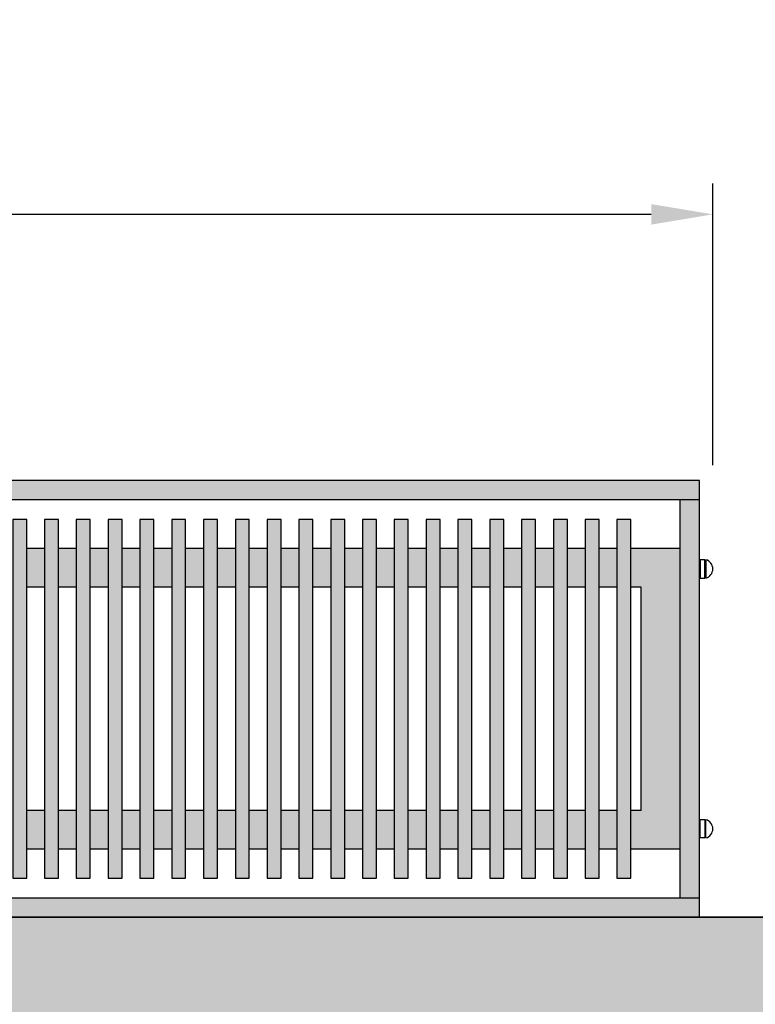
# Model space of a CAD drawing. Units: inches. Extents: x 3592 to 4861, y 1650 to 2243.
# Tile 14 of 30: x 4335 to 4365, y 1772 to 1812. Entities that reach past the tile are written whole.
import ezdxf

# ---------------------------------------------------------------- set-up
doc = ezdxf.new("R2010")
doc.units = ezdxf.units.IN
for name, color, linetype, lineweight in [('A-ANNO-DIMS', 2, 'Continuous', 13), ('A-FURN', 9, 'Continuous', 13), ('A-WALL', 7, 'Continuous', 35), ('estofado', 7, 'Continuous', 25)]:
    doc.layers.add(name, color=color, linetype=linetype, lineweight=lineweight)
doc.layers.add('A-WALL-PATT', color=252, linetype='Continuous', lineweight=13, true_color=0x939598)
doc.layers.add('MOBIL', color=7, linetype='Continuous')
doc.styles.get("Standard").update_dxf_attribs({"font": 'arial.ttf'})
doc.dimstyles.new('ISO-25', dxfattribs={"dimtxt": 9, "dimasz": 2.5, "dimexe": 1.25, "dimexo": 0.625, "dimtad": 1, "dimlunit": 3, "dimtxsty": 'Standard', "dimcen": 2.5, "dimadec": 0, "dimazin": 0, "dimtfac": 1, "dimtmove": 0, "dimatfit": 3, "dimfxl": 1, "dimarcsym": 0})

# ---------------------------------------------------------------- blocks, each defined once
blk = doc.blocks.new('Aparador Aido WV')
at = {"layer": 'MOBIL'}
h = blk.add_hatch(color=256, dxfattribs=at)
h.set_gradient(color1=(226, 228, 228), one_color=1, tint=1, name='CYLINDER')
h.paths.add_polyline_path([(0.9, -0.02), (0.9, 0), (-0.9, 0), (-0.9, -0.02)])
h = blk.add_hatch(color=256, dxfattribs=at)
h.set_gradient(color1=(226, 228, 228), one_color=1, tint=1)
h.paths.add_polyline_path([(-0.88, -0.02), (-0.9, -0.02), (-0.9, -0.43), (-0.88, -0.43)])
h = blk.add_hatch(color=256, dxfattribs=at)
h.set_gradient(color1=(106, 79, 62), color2=(55, 41, 32), one_color=1, tint=0.17)
h.paths.add_polyline_path([(-0.8151, -0.0402), (-0.8295, -0.0402), (-0.8295, -0.4098), (-0.8151, -0.4098)])
h = blk.add_hatch(color=256, dxfattribs=at)
h.set_gradient(color1=(106, 79, 62), color2=(55, 41, 32), one_color=1, tint=0.17)
h.paths.add_polyline_path([(-0.7967, -0.0402), (-0.7967, -0.4098), (-0.7823, -0.4098), (-0.7823, -0.0402)])
h = blk.add_hatch(color=256, dxfattribs=at)
h.set_gradient(color1=(106, 79, 62), color2=(55, 41, 32), one_color=1, tint=0.17)
h.paths.add_polyline_path([(-0.764, -0.0402), (-0.764, -0.4098), (-0.7496, -0.4098), (-0.7496, -0.0402)])
h = blk.add_hatch(color=256, dxfattribs=at)
h.set_gradient(color1=(106, 79, 62), color2=(55, 41, 32), one_color=1, tint=0.17)
h.paths.add_polyline_path([(-0.7312, -0.0402), (-0.7312, -0.4098), (-0.7168, -0.4098), (-0.7168, -0.0402)])
h = blk.add_hatch(color=256, dxfattribs=at)
h.set_gradient(color1=(106, 79, 62), color2=(55, 41, 32), one_color=1, tint=0.17)
h.paths.add_polyline_path([(-0.6985, -0.0402), (-0.6985, -0.4098), (-0.6841, -0.4098), (-0.6841, -0.0402)])
h = blk.add_hatch(color=256, dxfattribs=at)
h.set_gradient(color1=(106, 79, 62), color2=(55, 41, 32), one_color=1, tint=0.17)
h.paths.add_polyline_path([(-0.6657, -0.0402), (-0.6657, -0.4098), (-0.6513, -0.4098), (-0.6513, -0.0402)])
h = blk.add_hatch(color=256, dxfattribs=at)
h.set_gradient(color1=(106, 79, 62), color2=(55, 41, 32), one_color=1, tint=0.17)
h.paths.add_polyline_path([(-0.633, -0.0402), (-0.633, -0.4098), (-0.6186, -0.4098), (-0.6186, -0.0402)])
h = blk.add_hatch(color=256, dxfattribs=at)
h.set_gradient(color1=(106, 79, 62), color2=(55, 41, 32), one_color=1, tint=0.17)
h.paths.add_polyline_path([(-0.6002, -0.0402), (-0.6002, -0.4098), (-0.5858, -0.4098), (-0.5858, -0.0402)])
h = blk.add_hatch(color=256, dxfattribs=at)
h.set_gradient(color1=(106, 79, 62), color2=(55, 41, 32), one_color=1, tint=0.17)
h.paths.add_polyline_path([(-0.5675, -0.4098), (-0.5531, -0.4098), (-0.5531, -0.0402), (-0.5675, -0.0402)])
h = blk.add_hatch(color=256, dxfattribs=at)
h.set_gradient(color1=(106, 79, 62), color2=(55, 41, 32), one_color=1, tint=0.17)
h.paths.add_polyline_path([(-0.5347, -0.0402), (-0.5347, -0.4098), (-0.5203, -0.4098), (-0.5203, -0.0402)])
h = blk.add_hatch(color=256, dxfattribs=at)
h.set_gradient(color1=(106, 79, 62), color2=(55, 41, 32), one_color=1, tint=0.17)
h.paths.add_polyline_path([(-0.5019, -0.0402), (-0.5019, -0.4098), (-0.4876, -0.4098), (-0.4876, -0.0402)])
h = blk.add_hatch(color=256, dxfattribs=at)
h.set_gradient(color1=(106, 79, 62), color2=(55, 41, 32), one_color=1, tint=0.17)
h.paths.add_polyline_path([(-0.4692, -0.0402), (-0.4692, -0.4098), (-0.4548, -0.4098), (-0.4548, -0.0402)])
h = blk.add_hatch(color=256, dxfattribs=at)
h.set_gradient(color1=(106, 79, 62), color2=(55, 41, 32), one_color=1, tint=0.17)
h.paths.add_polyline_path([(-0.4364, -0.0402), (-0.4364, -0.4098), (-0.4221, -0.4098), (-0.4221, -0.0402)])
h = blk.add_hatch(color=256, dxfattribs=at)
h.set_gradient(color1=(106, 79, 62), color2=(55, 41, 32), one_color=1, tint=0.17)
h.paths.add_polyline_path([(-0.4037, -0.0402), (-0.4037, -0.4098), (-0.3893, -0.4098), (-0.3893, -0.0402)])
h = blk.add_hatch(color=256, dxfattribs=at)
h.set_gradient(color1=(106, 79, 62), color2=(55, 41, 32), one_color=1, tint=0.17)
h.paths.add_polyline_path([(-0.3709, -0.0402), (-0.3709, -0.4098), (-0.3566, -0.4098), (-0.3566, -0.0402)])
h = blk.add_hatch(color=256, dxfattribs=at)
h.set_gradient(color1=(106, 79, 62), color2=(55, 41, 32), one_color=1, tint=0.17)
h.paths.add_polyline_path([(-0.3382, -0.0402), (-0.3382, -0.4098), (-0.3238, -0.4098), (-0.3238, -0.0402)])
h = blk.add_hatch(color=256, dxfattribs=at)
h.set_gradient(color1=(106, 79, 62), color2=(55, 41, 32), one_color=1, tint=0.17)
h.paths.add_polyline_path([(-0.3054, -0.0402), (-0.3054, -0.4098), (-0.2911, -0.4098), (-0.2911, -0.0402)])
h = blk.add_hatch(color=256, dxfattribs=at)
h.set_gradient(color1=(106, 79, 62), color2=(55, 41, 32), one_color=1, tint=0.17)
h.paths.add_polyline_path([(-0.2727, -0.0402), (-0.2727, -0.4098), (-0.2583, -0.4098), (-0.2583, -0.0402)])
h = blk.add_hatch(color=256, dxfattribs=at)
h.set_gradient(color1=(106, 79, 62), color2=(55, 41, 32), one_color=1, tint=0.17)
h.paths.add_polyline_path([(-0.2399, -0.0402), (-0.2399, -0.4098), (-0.2256, -0.4098), (-0.2256, -0.0402)])
h = blk.add_hatch(color=256, dxfattribs=at)
h.set_gradient(color1=(106, 79, 62), color2=(55, 41, 32), one_color=1, tint=0.17)
h.paths.add_polyline_path([(-0.2072, -0.4098), (-0.1928, -0.4098), (-0.1928, -0.0402), (-0.2072, -0.0402)])
h = blk.add_hatch(color=256, dxfattribs=at)
h.set_gradient(color1=(106, 79, 62), color2=(157, 117, 92), one_color=1, tint=0.49)
h.paths.add_polyline_path([(-0.84, -0.11), (-0.8295, -0.11), (-0.8295, -0.07), (-0.88, -0.07), (-0.88, -0.38), (-0.8295, -0.38), (-0.8295, -0.34), (-0.84, -0.34)])
h = blk.add_hatch(color=256, dxfattribs=at)
h.set_gradient(color1=(106, 79, 62), color2=(157, 117, 92), one_color=1, tint=0.49)
h.paths.add_polyline_path([(-0.7967, -0.07), (-0.8151, -0.07), (-0.8151, -0.11), (-0.7967, -0.11)])
h = blk.add_hatch(color=256, dxfattribs=at)
h.set_gradient(color1=(106, 79, 62), color2=(157, 117, 92), one_color=1, tint=0.49)
h.paths.add_polyline_path([(-0.764, -0.07), (-0.7823, -0.07), (-0.7823, -0.11), (-0.764, -0.11)])
h = blk.add_hatch(color=256, dxfattribs=at)
h.set_gradient(color1=(106, 79, 62), color2=(157, 117, 92), one_color=1, tint=0.49)
h.paths.add_polyline_path([(-0.7312, -0.07), (-0.7496, -0.07), (-0.7496, -0.11), (-0.7312, -0.11)])
h = blk.add_hatch(color=256, dxfattribs=at)
h.set_gradient(color1=(106, 79, 62), color2=(157, 117, 92), one_color=1, tint=0.49)
h.paths.add_polyline_path([(-0.6985, -0.07), (-0.7168, -0.07), (-0.7168, -0.11), (-0.6985, -0.11)])
h = blk.add_hatch(color=256, dxfattribs=at)
h.set_gradient(color1=(106, 79, 62), color2=(157, 117, 92), one_color=1, tint=0.49)
h.paths.add_polyline_path([(-0.6657, -0.07), (-0.6841, -0.07), (-0.6841, -0.11), (-0.6657, -0.11)])
h = blk.add_hatch(color=256, dxfattribs=at)
h.set_gradient(color1=(106, 79, 62), color2=(157, 117, 92), one_color=1, tint=0.49)
h.paths.add_polyline_path([(-0.633, -0.07), (-0.6513, -0.07), (-0.6513, -0.11), (-0.633, -0.11)])
h = blk.add_hatch(color=256, dxfattribs=at)
h.set_gradient(color1=(106, 79, 62), color2=(157, 117, 92), one_color=1, tint=0.49)
h.paths.add_polyline_path([(-0.6002, -0.07), (-0.6186, -0.07), (-0.6186, -0.11), (-0.6002, -0.11)])
h = blk.add_hatch(color=256, dxfattribs=at)
h.set_gradient(color1=(106, 79, 62), color2=(157, 117, 92), one_color=1, tint=0.49)
h.paths.add_polyline_path([(-0.5675, -0.07), (-0.5858, -0.07), (-0.5858, -0.11), (-0.5675, -0.11)])
h = blk.add_hatch(color=256, dxfattribs=at)
h.set_gradient(color1=(106, 79, 62), color2=(157, 117, 92), one_color=1, tint=0.49)
h.paths.add_polyline_path([(-0.5347, -0.07), (-0.5531, -0.07), (-0.5531, -0.11), (-0.5347, -0.11)])
h = blk.add_hatch(color=256, dxfattribs=at)
h.set_gradient(color1=(106, 79, 62), color2=(157, 117, 92), one_color=1, tint=0.49)
h.paths.add_polyline_path([(-0.5019, -0.07), (-0.5203, -0.07), (-0.5203, -0.11), (-0.5019, -0.11)])
h = blk.add_hatch(color=256, dxfattribs=at)
h.set_gradient(color1=(106, 79, 62), color2=(157, 117, 92), one_color=1, tint=0.49)
h.paths.add_polyline_path([(-0.4692, -0.07), (-0.4876, -0.07), (-0.4876, -0.11), (-0.4692, -0.11)])
h = blk.add_hatch(color=256, dxfattribs=at)
h.set_gradient(color1=(106, 79, 62), color2=(157, 117, 92), one_color=1, tint=0.49)
h.paths.add_polyline_path([(-0.4364, -0.07), (-0.4548, -0.07), (-0.4548, -0.11), (-0.4364, -0.11)])
h = blk.add_hatch(color=256, dxfattribs=at)
h.set_gradient(color1=(106, 79, 62), color2=(157, 117, 92), one_color=1, tint=0.49)
h.paths.add_polyline_path([(-0.4037, -0.07), (-0.4221, -0.07), (-0.4221, -0.11), (-0.4037, -0.11)])
h = blk.add_hatch(color=256, dxfattribs=at)
h.set_gradient(color1=(106, 79, 62), color2=(157, 117, 92), one_color=1, tint=0.49)
h.paths.add_polyline_path([(-0.3709, -0.07), (-0.3893, -0.07), (-0.3893, -0.11), (-0.3709, -0.11)])
h = blk.add_hatch(color=256, dxfattribs=at)
h.set_gradient(color1=(106, 79, 62), color2=(157, 117, 92), one_color=1, tint=0.49)
h.paths.add_polyline_path([(-0.3382, -0.07), (-0.3566, -0.07), (-0.3566, -0.11), (-0.3382, -0.11)])
h = blk.add_hatch(color=256, dxfattribs=at)
h.set_gradient(color1=(106, 79, 62), color2=(157, 117, 92), one_color=1, tint=0.49)
h.paths.add_polyline_path([(-0.3054, -0.07), (-0.3238, -0.07), (-0.3238, -0.11), (-0.3054, -0.11)])
h = blk.add_hatch(color=256, dxfattribs=at)
h.set_gradient(color1=(106, 79, 62), color2=(157, 117, 92), one_color=1, tint=0.49)
h.paths.add_polyline_path([(-0.2727, -0.07), (-0.2911, -0.07), (-0.2911, -0.11), (-0.2727, -0.11)])
h = blk.add_hatch(color=256, dxfattribs=at)
h.set_gradient(color1=(106, 79, 62), color2=(157, 117, 92), one_color=1, tint=0.49)
h.paths.add_polyline_path([(-0.2399, -0.07), (-0.2583, -0.07), (-0.2583, -0.11), (-0.2399, -0.11)])
h = blk.add_hatch(color=256, dxfattribs=at)
h.set_gradient(color1=(106, 79, 62), color2=(157, 117, 92), one_color=1, tint=0.49)
h.paths.add_polyline_path([(-0.2072, -0.07), (-0.2256, -0.07), (-0.2256, -0.11), (-0.2072, -0.11)])
h = blk.add_hatch(color=256, dxfattribs=at)
h.set_gradient(color1=(106, 79, 62), color2=(157, 117, 92), one_color=1, tint=0.49)
h.paths.add_polyline_path([(-0.7967, -0.34), (-0.8151, -0.34), (-0.8151, -0.38), (-0.7967, -0.38)])
h = blk.add_hatch(color=256, dxfattribs=at)
h.set_gradient(color1=(106, 79, 62), color2=(157, 117, 92), one_color=1, tint=0.49)
h.paths.add_polyline_path([(-0.764, -0.34), (-0.7823, -0.34), (-0.7823, -0.38), (-0.764, -0.38)])
h = blk.add_hatch(color=256, dxfattribs=at)
h.set_gradient(color1=(106, 79, 62), color2=(157, 117, 92), one_color=1, tint=0.49)
h.paths.add_polyline_path([(-0.7312, -0.34), (-0.7496, -0.34), (-0.7496, -0.38), (-0.7312, -0.38)])
h = blk.add_hatch(color=256, dxfattribs=at)
h.set_gradient(color1=(106, 79, 62), color2=(157, 117, 92), one_color=1, tint=0.49)
h.paths.add_polyline_path([(-0.6985, -0.34), (-0.7168, -0.34), (-0.7168, -0.38), (-0.6985, -0.38)])
h = blk.add_hatch(color=256, dxfattribs=at)
h.set_gradient(color1=(106, 79, 62), color2=(157, 117, 92), one_color=1, tint=0.49)
h.paths.add_polyline_path([(-0.6657, -0.34), (-0.6841, -0.34), (-0.6841, -0.38), (-0.6657, -0.38)])
h = blk.add_hatch(color=256, dxfattribs=at)
h.set_gradient(color1=(106, 79, 62), color2=(157, 117, 92), one_color=1, tint=0.49)
h.paths.add_polyline_path([(-0.633, -0.34), (-0.6513, -0.34), (-0.6513, -0.38), (-0.633, -0.38)])
h = blk.add_hatch(color=256, dxfattribs=at)
h.set_gradient(color1=(106, 79, 62), color2=(157, 117, 92), one_color=1, tint=0.49)
h.paths.add_polyline_path([(-0.6002, -0.34), (-0.6186, -0.34), (-0.6186, -0.38), (-0.6002, -0.38)])
h = blk.add_hatch(color=256, dxfattribs=at)
h.set_gradient(color1=(106, 79, 62), color2=(157, 117, 92), one_color=1, tint=0.49)
h.paths.add_polyline_path([(-0.5675, -0.34), (-0.5858, -0.34), (-0.5858, -0.38), (-0.5675, -0.38)])
h = blk.add_hatch(color=256, dxfattribs=at)
h.set_gradient(color1=(106, 79, 62), color2=(157, 117, 92), one_color=1, tint=0.49)
h.paths.add_polyline_path([(-0.5347, -0.34), (-0.5531, -0.34), (-0.5531, -0.38), (-0.5347, -0.38)])
h = blk.add_hatch(color=256, dxfattribs=at)
h.set_gradient(color1=(106, 79, 62), color2=(157, 117, 92), one_color=1, tint=0.49)
h.paths.add_polyline_path([(-0.5019, -0.34), (-0.5203, -0.34), (-0.5203, -0.38), (-0.5019, -0.38)])
h = blk.add_hatch(color=256, dxfattribs=at)
h.set_gradient(color1=(106, 79, 62), color2=(157, 117, 92), one_color=1, tint=0.49)
h.paths.add_polyline_path([(-0.4692, -0.34), (-0.4876, -0.34), (-0.4876, -0.38), (-0.4692, -0.38)])
h = blk.add_hatch(color=256, dxfattribs=at)
h.set_gradient(color1=(106, 79, 62), color2=(157, 117, 92), one_color=1, tint=0.49)
h.paths.add_polyline_path([(-0.4364, -0.34), (-0.4548, -0.34), (-0.4548, -0.38), (-0.4364, -0.38)])
h = blk.add_hatch(color=256, dxfattribs=at)
h.set_gradient(color1=(106, 79, 62), color2=(157, 117, 92), one_color=1, tint=0.49)
h.paths.add_polyline_path([(-0.4037, -0.34), (-0.4221, -0.34), (-0.4221, -0.38), (-0.4037, -0.38)])
h = blk.add_hatch(color=256, dxfattribs=at)
h.set_gradient(color1=(106, 79, 62), color2=(157, 117, 92), one_color=1, tint=0.49)
h.paths.add_polyline_path([(-0.3709, -0.34), (-0.3893, -0.34), (-0.3893, -0.38), (-0.3709, -0.38)])
h = blk.add_hatch(color=256, dxfattribs=at)
h.set_gradient(color1=(106, 79, 62), color2=(157, 117, 92), one_color=1, tint=0.49)
h.paths.add_polyline_path([(-0.3382, -0.34), (-0.3566, -0.34), (-0.3566, -0.38), (-0.3382, -0.38)])
h = blk.add_hatch(color=256, dxfattribs=at)
h.set_gradient(color1=(106, 79, 62), color2=(157, 117, 92), one_color=1, tint=0.49)
h.paths.add_polyline_path([(-0.3054, -0.34), (-0.3238, -0.34), (-0.3238, -0.38), (-0.3054, -0.38)])
h = blk.add_hatch(color=256, dxfattribs=at)
h.set_gradient(color1=(106, 79, 62), color2=(157, 117, 92), one_color=1, tint=0.49)
h.paths.add_polyline_path([(-0.2727, -0.34), (-0.2911, -0.34), (-0.2911, -0.38), (-0.2727, -0.38)])
h = blk.add_hatch(color=256, dxfattribs=at)
h.set_gradient(color1=(106, 79, 62), color2=(157, 117, 92), one_color=1, tint=0.49)
h.paths.add_polyline_path([(-0.2399, -0.34), (-0.2583, -0.34), (-0.2583, -0.38), (-0.2399, -0.38)])
h = blk.add_hatch(color=256, dxfattribs=at)
h.set_gradient(color1=(106, 79, 62), color2=(157, 117, 92), one_color=1, tint=0.49)
h.paths.add_polyline_path([(-0.2072, -0.34), (-0.2256, -0.34), (-0.2256, -0.38), (-0.2072, -0.38)])
h = blk.add_hatch(color=256, dxfattribs=at)
h.set_gradient(color1=(226, 228, 228), one_color=1, tint=1, name='CYLINDER')
h.paths.add_polyline_path([(0.9, -0.45), (0.9, -0.43), (-0.9, -0.43), (-0.9, -0.45)])
at = {"layer": 'estofado', "ltscale": 0.5}
for p, q in [((-0.88, -0.07), (-0.8295, -0.07)), ((-0.8151, -0.07), (-0.7967, -0.07)), ((-0.7823, -0.07), (-0.764, -0.07)), ((-0.7496, -0.07), (-0.7312, -0.07)), ((-0.7168, -0.07), (-0.6985, -0.07)), ((-0.6841, -0.07), (-0.6657, -0.07)), ((-0.6513, -0.07), (-0.633, -0.07)), ((-0.6186, -0.07), (-0.6002, -0.07)), ((-0.5858, -0.07), (-0.5675, -0.07)), ((-0.5531, -0.07), (-0.5347, -0.07)), ((-0.5203, -0.07), (-0.5019, -0.07)), ((-0.4876, -0.07), (-0.4692, -0.07)), ((-0.4548, -0.07), (-0.4364, -0.07)), ((-0.4221, -0.07), (-0.4037, -0.07)), ((-0.3893, -0.07), (-0.3709, -0.07)), ((-0.3566, -0.07), (-0.3382, -0.07)), ((-0.3238, -0.07), (-0.3054, -0.07)), ((-0.2911, -0.07), (-0.2727, -0.07)), ((-0.2583, -0.07), (-0.2399, -0.07)), ((-0.2256, -0.07), (-0.2072, -0.07)), ((-0.9067, -0.0817), (-0.9067, -0.1006)), ((-0.84, -0.11), (-0.84, -0.34)), ((-0.84, -0.11), (-0.8295, -0.11)), ((-0.8151, -0.11), (-0.7967, -0.11)), ((-0.7823, -0.11), (-0.764, -0.11)), ((-0.7496, -0.11), (-0.7312, -0.11)), ((-0.7168, -0.11), (-0.6985, -0.11)), ((-0.6841, -0.11), (-0.6657, -0.11)), ((-0.6513, -0.11), (-0.633, -0.11)), ((-0.6186, -0.11), (-0.6002, -0.11)), ((-0.5858, -0.11), (-0.5675, -0.11)), ((-0.5531, -0.11), (-0.5347, -0.11)), ((-0.5203, -0.11), (-0.5019, -0.11)), ((-0.4876, -0.11), (-0.4692, -0.11)), ((-0.4548, -0.11), (-0.4364, -0.11)), ((-0.4221, -0.11), (-0.4037, -0.11)), ((-0.3893, -0.11), (-0.3709, -0.11)), ((-0.3566, -0.11), (-0.3382, -0.11)), ((-0.3238, -0.11), (-0.3054, -0.11)), ((-0.2911, -0.11), (-0.2727, -0.11)), ((-0.2583, -0.11), (-0.2399, -0.11)), ((-0.2256, -0.11), (-0.2072, -0.11)), ((-0.84, -0.34), (-0.8295, -0.34)), ((-0.8151, -0.34), (-0.7967, -0.34)), ((-0.7823, -0.34), (-0.764, -0.34)), ((-0.7496, -0.34), (-0.7312, -0.34)), ((-0.7168, -0.34), (-0.6985, -0.34)), ((-0.6841, -0.34), (-0.6657, -0.34)), ((-0.6513, -0.34), (-0.633, -0.34)), ((-0.6186, -0.34), (-0.6002, -0.34)), ((-0.5858, -0.34), (-0.5675, -0.34)), ((-0.5531, -0.34), (-0.5347, -0.34)), ((-0.5203, -0.34), (-0.5019, -0.34)), ((-0.4876, -0.34), (-0.4692, -0.34)), ((-0.4548, -0.34), (-0.4364, -0.34)), ((-0.4221, -0.34), (-0.4037, -0.34)), ((-0.3893, -0.34), (-0.3709, -0.34)), ((-0.3566, -0.34), (-0.3382, -0.34)), ((-0.3238, -0.34), (-0.3054, -0.34)), ((-0.2911, -0.34), (-0.2727, -0.34)), ((-0.2583, -0.34), (-0.2399, -0.34)), ((-0.2256, -0.34), (-0.2072, -0.34)), ((-0.9067, -0.3683), (-0.9067, -0.3494)), ((-0.88, -0.38), (-0.8295, -0.38)), ((-0.84, -0.38), (-0.8295, -0.38)), ((-0.8151, -0.38), (-0.7967, -0.38)), ((-0.7823, -0.38), (-0.764, -0.38)), ((-0.7496, -0.38), (-0.7312, -0.38)), ((-0.7168, -0.38), (-0.6985, -0.38)), ((-0.6841, -0.38), (-0.6657, -0.38)), ((-0.6513, -0.38), (-0.633, -0.38)), ((-0.6186, -0.38), (-0.6002, -0.38)), ((-0.5858, -0.38), (-0.5675, -0.38)), ((-0.5531, -0.38), (-0.5347, -0.38)), ((-0.5203, -0.38), (-0.5019, -0.38)), ((-0.4876, -0.38), (-0.4692, -0.38)), ((-0.4548, -0.38), (-0.4364, -0.38)), ((-0.4221, -0.38), (-0.4037, -0.38)), ((-0.3893, -0.38), (-0.3709, -0.38)), ((-0.3566, -0.38), (-0.3382, -0.38)), ((-0.3238, -0.38), (-0.3054, -0.38)), ((-0.2911, -0.38), (-0.2727, -0.38)), ((-0.2583, -0.38), (-0.2399, -0.38)), ((-0.2256, -0.38), (-0.2072, -0.38))]:
    blk.add_line(p, q, dxfattribs=at)
for points in [[(-0.8295, -0.0402), (-0.8295, -0.4098), (-0.8151, -0.4098), (-0.8151, -0.0402)], [(-0.7967, -0.0402), (-0.7967, -0.4098), (-0.7823, -0.4098), (-0.7823, -0.0402)], [(-0.764, -0.0402), (-0.764, -0.4098), (-0.7496, -0.4098), (-0.7496, -0.0402)], [(-0.7312, -0.0402), (-0.7312, -0.4098), (-0.7168, -0.4098), (-0.7168, -0.0402)], [(-0.6985, -0.0402), (-0.6985, -0.4098), (-0.6841, -0.4098), (-0.6841, -0.0402)], [(-0.6657, -0.0402), (-0.6657, -0.4098), (-0.6513, -0.4098), (-0.6513, -0.0402)], [(-0.633, -0.0402), (-0.633, -0.4098), (-0.6186, -0.4098), (-0.6186, -0.0402)], [(-0.6002, -0.0402), (-0.6002, -0.4098), (-0.5858, -0.4098), (-0.5858, -0.0402)], [(-0.5675, -0.0402), (-0.5675, -0.4098), (-0.5531, -0.4098), (-0.5531, -0.0402)], [(-0.5347, -0.0402), (-0.5347, -0.4098), (-0.5203, -0.4098), (-0.5203, -0.0402)], [(-0.5019, -0.0402), (-0.5019, -0.4098), (-0.4876, -0.4098), (-0.4876, -0.0402)], [(-0.4692, -0.0402), (-0.4692, -0.4098), (-0.4548, -0.4098), (-0.4548, -0.0402)], [(-0.4364, -0.0402), (-0.4364, -0.4098), (-0.4221, -0.4098), (-0.4221, -0.0402)], [(-0.4037, -0.0402), (-0.4037, -0.4098), (-0.3893, -0.4098), (-0.3893, -0.0402)], [(-0.3709, -0.0402), (-0.3709, -0.4098), (-0.3566, -0.4098), (-0.3566, -0.0402)], [(-0.3382, -0.0402), (-0.3382, -0.4098), (-0.3238, -0.4098), (-0.3238, -0.0402)], [(-0.3054, -0.0402), (-0.3054, -0.4098), (-0.2911, -0.4098), (-0.2911, -0.0402)], [(-0.2727, -0.0402), (-0.2727, -0.4098), (-0.2583, -0.4098), (-0.2583, -0.0402)], [(-0.2399, -0.0402), (-0.2399, -0.4098), (-0.2256, -0.4098), (-0.2256, -0.0402)], [(-0.2072, -0.0402), (-0.2072, -0.4098), (-0.1928, -0.4098), (-0.1928, -0.0402)], [(-0.9054, -0.0817), (-0.9009, -0.0817), (-0.9009, -0.1006), (-0.9054, -0.1006)], [(-0.9054, -0.3683), (-0.9009, -0.3683), (-0.9009, -0.3494), (-0.9054, -0.3494)]]:
    blk.add_lwpolyline(points, close=True, dxfattribs=at)
for centre in [(-0.904, -0.0911), (-0.904, -0.3589)]:
    blk.add_arc(centre, 0.0098, 105.9849, 254.0151, dxfattribs=at)
at = {"layer": 'MOBIL'}
for p, q in [((0.9, -0.02), (-0.9, -0.02)), ((-0.88, -0.02), (-0.88, -0.43)), ((-0.9, -0.43), (0.9, -0.43))]:
    blk.add_line(p, q, dxfattribs=at)
blk.add_lwpolyline([(-0.9, -0.45), (0.9, -0.45), (0.9, 0), (-0.9, 0)], close=True, dxfattribs=at)
blk = doc.blocks.new('*D156')
at = {"layer": 'A-ANNO-DIMS', "color": 0, "lineweight": -2, "transparency": 16777216}
for p, q in [((4291.393, 1793.561), (4291.393, 1804.979)), ((4363.347, 1793.561), (4363.347, 1804.979)), ((4291.393, 1803.729), (4155.277, 1803.729)), ((4360.847, 1803.729), (4293.893, 1803.729))]:
    blk.add_line(p, q, dxfattribs=at)
at = {"layer": 'A-ANNO-DIMS', "color": 0, "transparency": 16777216}
for points in [[(4293.893, 1804.145), (4293.893, 1803.312), (4291.393, 1803.729)], [(4360.847, 1804.145), (4360.847, 1803.312), (4363.347, 1803.729)]]:
    blk.add_solid(points, dxfattribs=at)
at = {"layer": 'Defpoints', "color": 0, "transparency": 16777216}
for p in [(4291.393, 1803.729), (4291.393, 1792.936), (4363.347, 1792.936)]:
    blk.add_point(p, dxfattribs=at)
at = {"layer": 'A-ANNO-DIMS', "color": 0, "transparency": 16777216, "insert": (4222.085, 1809.01), "char_height": 9, "attachment_point": 5}
blk.add_mtext('SIDEBOARD 6\'-0" TYP.', dxfattribs=at)

msp = doc.modelspace()

# ---------------------------------------------------------------- hatches: boundary and pattern name
at = {"layer": 'A-WALL-PATT'}
h = msp.add_hatch(color=256, dxfattribs=at)
h.dxf.hatch_style = 1
h.paths.add_polyline_path([(4398.37, 2165.219), (4038.37, 2165.219), (4038.37, 1993.219), (4047.37, 1993.219), (4047.37, 2156.219), (4191.37, 2156.219), (4191.37, 2150.219), (4195.37, 2150.219), (4195.37, 2156.219), (4256.37, 2156.219), (4256.37, 2150.219), (4265.37, 2150.219), (4265.37, 2156.219), (4389.37, 2156.219), (4389.37, 2114.219), (4398.37, 2114.219)])
h.paths.add_polyline_path([(4265.37, 2102.219), (4256.37, 2102.219), (4256.37, 2096.219), (4195.37, 2096.219), (4195.37, 2102.219), (4191.37, 2102.219), (4191.37, 2020.219), (4195.37, 2020.219), (4195.37, 2087.219), (4256.37, 2087.219), (4256.37, 2020.219), (4306.37, 2020.219), (4306.37, 2024.219), (4265.37, 2024.219)], flags=17)
h.paths.add_polyline_path([(4398.37, 2066.219), (4389.37, 2066.219), (4389.37, 2024.219), (4348.37, 2024.219), (4348.37, 2020.219), (4389.37, 2020.219), (4389.37, 1989.719), (4398.37, 1989.719)])
h.paths.add_polyline_path([(4398.37, 1941.719), (4389.37, 1941.719), (4389.37, 1911.219), (4301.37, 1911.219), (4301.37, 1907.219), (4389.37, 1907.219), (4389.37, 1865.219), (4398.37, 1865.219)])
h.paths.add_polyline_path([(4398.37, 1817.219), (4389.37, 1817.219), (4389.37, 1775.219), (4265.37, 1775.219), (4265.37, 1911.219), (4256.37, 1911.219), (4256.37, 1817.219), (4220.87, 1817.219), (4220.87, 1808.219), (4256.37, 1808.219), (4256.37, 1766.219), (4389.37, 1766.219), (4389.37, 1694.219), (4256.37, 1694.219), (4256.37, 1685.219), (4398.37, 1685.219)])
h.paths.add_polyline_path([(4178.87, 1817.219), (4077.37, 1817.219), (4077.37, 1808.219), (4178.87, 1808.219)])
h.paths.add_polyline_path([(4111.37, 2020.219), (4155.37, 2020.219), (4155.37, 2024.219), (4077.37, 2024.219), (4077.37, 2020.219), (4107.37, 2020.219), (4107.37, 1942.219), (4047.37, 1942.219), (4047.37, 1969.219), (4038.37, 1969.219), (4038.37, 1911.219), (4047.37, 1911.219), (4047.37, 1938.219), (4107.37, 1938.219), (4107.37, 1860.219), (4077.37, 1860.219), (4077.37, 1856.219), (4111.37, 1856.219)])
h.paths.add_polyline_path([(4047.37, 1887.219), (4038.37, 1887.219), (4038.37, 1685.219), (4152.37, 1685.219), (4152.37, 1715.219), (4143.37, 1715.219), (4143.37, 1694.219), (4047.37, 1694.219)])
h.paths.add_polyline_path([(4152.37, 1772.219), (4143.37, 1772.219), (4143.37, 1751.219), (4152.37, 1751.219)], flags=17)

# ---------------------------------------------------------------- linework, layer by layer
at = {"layer": 'A-WALL'}
msp.add_line((4389.37, 1775.219), (4265.37, 1775.219), dxfattribs=at)

# ---------------------------------------------------------------- block references
at = {"layer": 'A-FURN', "xscale": 39.3701, "yscale": 39.3701, "zscale": 39.3701, "rotation": 180}
msp.add_blockref('Aparador Aido WV', (4327.37, 1775.219), dxfattribs=at)

# ---------------------------------------------------------------- dimensions: what is measured, and where the dimension line sits
at = {"layer": 'A-ANNO-DIMS'}
dim = msp.add_linear_dim(base=(4291.393, 1803.729), p1=(4363.347, 1792.936), p2=(4291.393, 1792.936), angle=180, text='SIDEBOARD <> TYP.', dimstyle='ISO-25', override={"dimdec": 1, "dimlfac": 1, "dimrnd": 0, "dimzin": 1, "dimdsep": 46, "dimlunit": 4, "dimfrac": 2}, dxfattribs=at)
dim.commit()
dim.dimension.update_dxf_attribs({"geometry": '*D156', "text_midpoint": (4222.085, 1809.01)})

doc.saveas('drawing.dxf')
